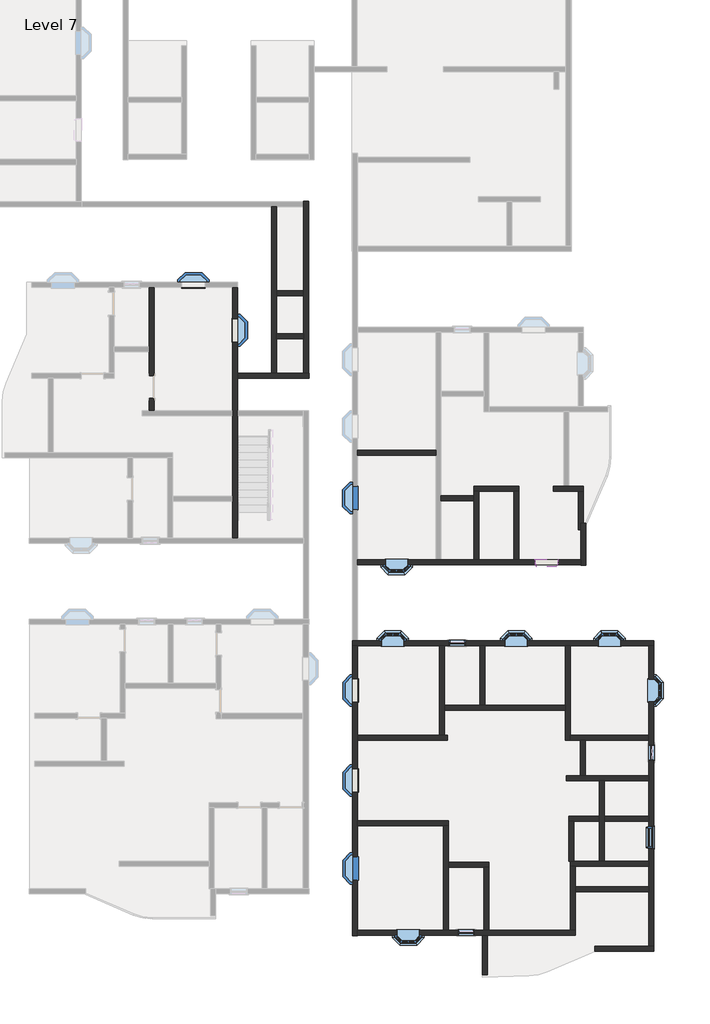
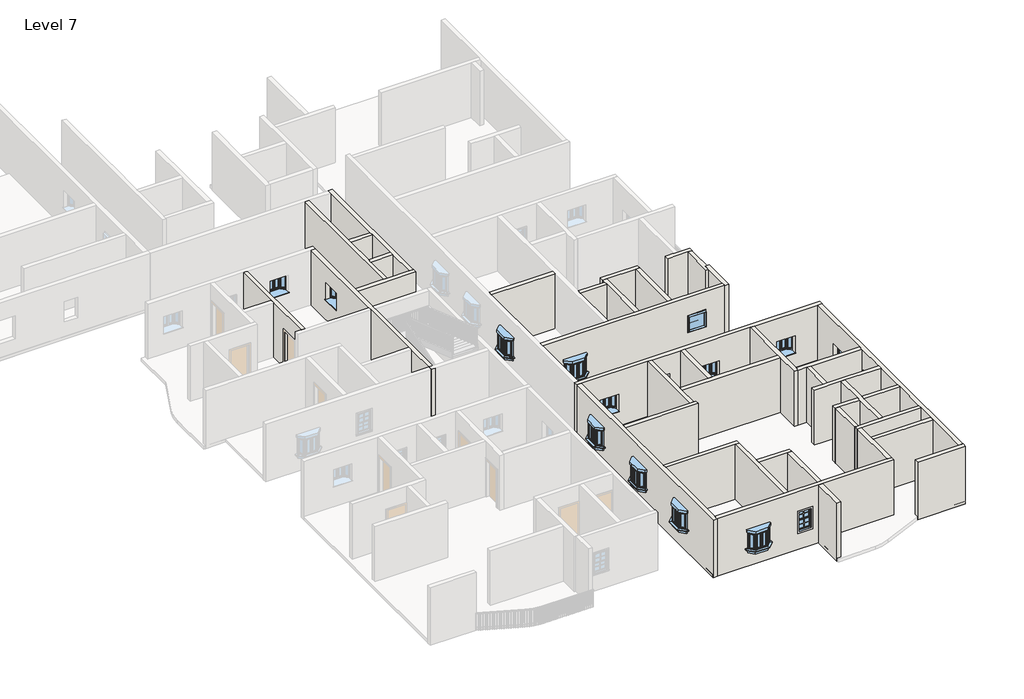
# One storey, part 2 of 14: 40 walls, 17 windows.
# Revit data of these elements (continued)
# Element 47 (IfcWindow, "910x910mm") (continued)
#   Mark = "383"
#   Phase Created = New Construction
#   Materials on its faces: "Window Frame", "Glass"
# Element 48 (IfcWindow, "910x910mm")
#   Mark = "384"
#   Phase Created = New Construction
#   Materials on its faces: "Window Frame", "Glass"
# Element 49 (IfcWindow, "910x910mm")
#   Mark = "385"
#   Phase Created = New Construction
#   Materials on its faces: "Window Frame", "Glass"
# Element 50 (IfcWindow, "910x910mm")
#   Mark = "386"
#   Phase Created = New Construction
#   Materials on its faces: "Window Frame", "Glass"
# Element 51 (IfcWindow, "910x910mm")
#   Mark = "387"
#   Phase Created = New Construction
#   Materials on its faces: "Window Frame", "Glass"
# Element 52 (IfcWindow, "910x910mm")
#   Mark = "388"
#   Phase Created = New Construction
#   Materials on its faces: "Window Frame", "Glass"
# Element 53 (IfcWindow, "Window-Double-Hung : 26\" x 42\"")
#   Mark = "411"
#   Window Inset = 0' - 0"
#   Interior Wall Closure = 0' - 1 1/2"
#   Frame Extension = 0' - 1 1/4"
#   Exterior Wall Closure = 0' - 0 1/2"
#   Interior Trim Visibility = yes
#   Indicator Visibility = yes
#   Exterior Trim Visibility = yes
#   Phase Created = New Construction
#   Materials on its faces: "Wood - Stained", "Glass", "Clad - White"
# Element 54 (IfcWindow, "Window-Double-Hung : 26\" x 42\"")
#   Mark = "412"
#   Window Inset = 0' - 0"
#   Interior Wall Closure = 0' - 1 1/2"
#   Frame Extension = 0' - 1 1/4"
#   Exterior Wall Closure = 0' - 0 1/2"
#   Interior Trim Visibility = yes
#   Indicator Visibility = yes
#   Exterior Trim Visibility = yes
#   Phase Created = New Construction
#   Materials on its faces: "Wood - Stained", "Glass", "Clad - White"
# Element 55 (IfcWindow, "Window-Double-Hung : 26\" x 42\"")
#   Mark = "413"
#   Window Inset = 0' - 0"
#   Interior Wall Closure = 0' - 1 1/2"
#   Frame Extension = 0' - 1 1/4"
#   Exterior Wall Closure = 0' - 0 1/2"
#   Interior Trim Visibility = yes
#   Indicator Visibility = yes
#   Exterior Trim Visibility = yes
#   Phase Created = New Construction
#   Materials on its faces: "Wood - Stained", "Glass", "Clad - White"
# Element 56 (IfcWindow, "Windows_Sgl_w-Glazing_Bars : 910x910mm")
#   Mark = "401"
#   Phase Created = New Construction
#   Materials on its faces: "Window Frame", "Glass"
# Element 57 (IfcWindow, "Windows_Sgl_w-Glazing_Bars : 910x910mm")
#   Mark = "400"
#   Phase Created = New Construction
#   Materials on its faces: "Window Frame", "Glass"
# Materials
#   "Window Frame": colour RGB 249 249 249, transparency 0
#   "Glass": class "Glass", colour RGB 0 128 192, transparency 0.75, Description = "Soda Lime Glass", Cost = 0
#   "Wood - Stained": class "Wood", colour RGB 224 178 126, transparency 0, Cost = 0
#   "Clad - White": class "Wood", colour RGB 242 242 238, transparency 0, Cost = 0
#   "Default Wall": colour RGB 128 128 128, transparency 0, Cost = 0
#   "Door - Frame": colour RGB 118 70 51, transparency 0, Cost = 0
#   "Earth": class "Generic", colour RGB 97 75 62, transparency 0, Description = "Soil", Cost = 0
#   "Carpet (1)": class "Carpet", colour RGB 124 80 67, transparency 0, Description = "Interior finish", Cost = 0
#   "Acoustic Ceiling Tile 24 x 24": class "Generic", colour RGB 232 232 232, transparency 0, Description = "Acoustic Ceiling Tile 24 x 24", Cost = 0
